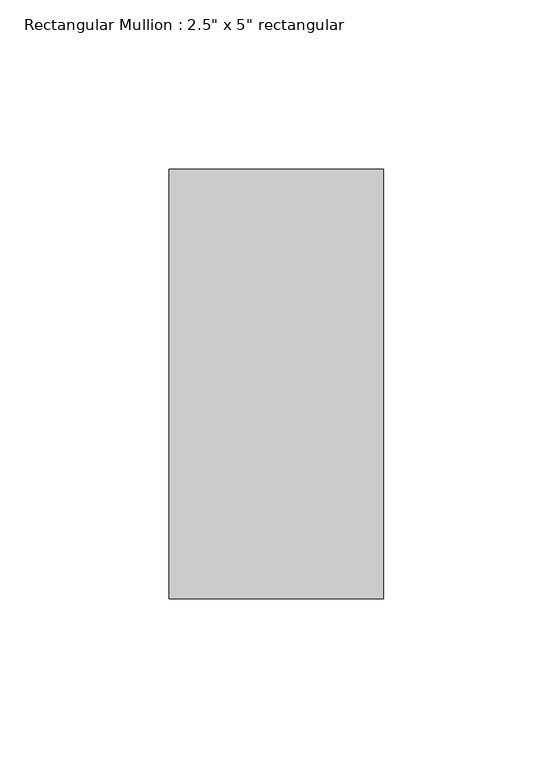
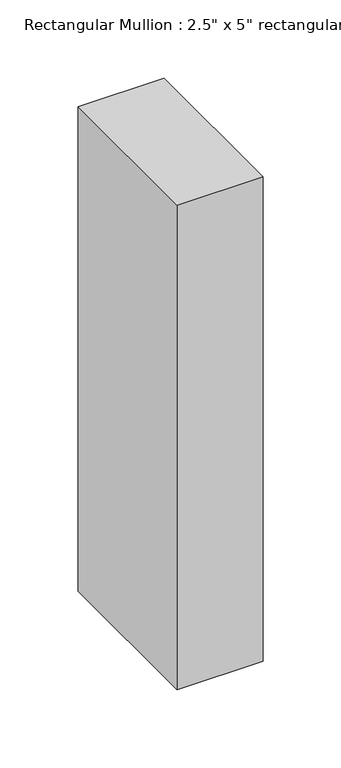
"""IFC4 building model written with IfcOpenShell, lengths in millimetres: member geometry."""

from ifc_helpers import new_model, si_unit, frame, origin, place, context, project, spatial, polyline, outline, extrude, source, transform, mapped, element, save


def member_35330a42(model_context):
    return source(origin(), model_context, "Body", "SweptSolid", [
        extrude(outline(polyline([(0.0, 63.5), (0.0, -63.5), (-63.5, -63.5), (-63.5, 63.5), (0.0, 63.5)])), frame((0.0, 0.0, -378.8833333), z_axis=(0.0, 0.0, 1.0), x_axis=(1.0, 0.0, 0.0)), (0.0, 0.0, 1.0), 378.8833333),
    ])


if __name__ == "__main__":
    model = new_model("IFC4")
    model_context = context("Model", 3, world=origin())
    ifc_project = project(units=[si_unit("LENGTHUNIT", "METRE", prefix="MILLI")], contexts=[model_context])
    site = spatial("IfcSite", under=ifc_project)
    building = spatial("IfcBuilding", under=site)
    placement = place(None, origin())
    member_shape = member_35330a42(model_context)
    element("IfcMember", 1, ObjectType="Rectangular Mullion : 2.5\" x 5\" rectangular", at=placement, inside=building, context=model_context, shape_type="MappedRepresentation", body=[
        mapped(member_shape, transform((0.0, 0.0, 0.0), x_axis=(1.0, 0.0, 0.0), y_axis=(0.0, 1.0, 0.0), z_axis=(0.0, 0.0, 1.0))),
    ])
    save(model, "model.ifc")

# Revit data of these elements
# Type "Rectangular Mullion : 2.5\" x 5\" rectangular"
#   built-in parameter 1007304 = 0.416667 (stored number, unit not read)
#   built-in parameter 1007301 = 0.104167 (stored number, unit not read)
#   built-in parameter 1007300 = 0.104167 (stored number, unit not read)
